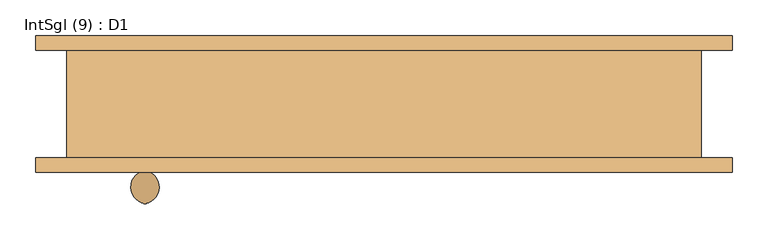
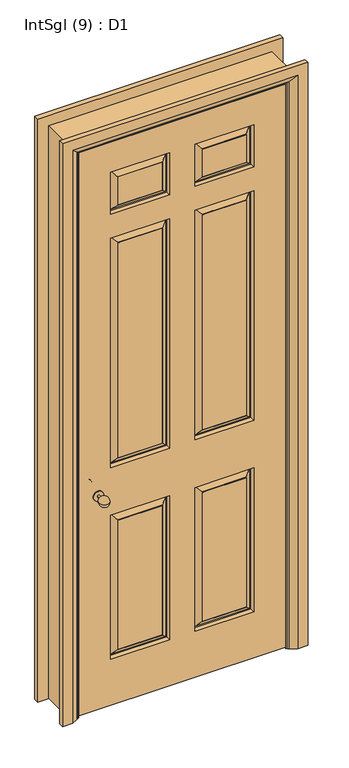
"""IFC4 building model written with IfcOpenShell, lengths in millimetres: door geometry, IntSgl (9) : D1."""

from ifc_helpers import new_model, si_unit, point, frame, origin, place, context, project, spatial, polyline, circle_curve, ellipse_curve, trimmed, outline, extrude, faceted_brep, source, transform, mapped, element, save
from ifc_brep_helpers import plane_surface, cylinder_surface, revolved_surface, advanced_brep


def intsgl_9_d1_ea64c5f3(model_context):
    return source(origin(), model_context, "Body", "SolidModel", [
        advanced_brep(
        [(-328.0, -18.0, 900.0), (-338.0, -18.0, 900.0), (-333.0, 26.437411, 900.0), (-328.0, -33.0, 900.0), (-338.0, -33.0, 900.0), (-353.0, -37.0, 900.0), (-313.0, -37.0, 900.0), (-353.0, -33.0, 900.0), (-313.0, -33.0, 900.0)],
        [
            (0, 1, circle_curve(frame((-333.0, -18.0, 900.0), z_axis=(0.0, 1.0, 0.0), x_axis=(-1.0, 0.0, 0.0)), 5.0)),
            (1, 2, circle_curve(frame((-329.8115138, 3.5786495, 900.0), z_axis=(0.0, 0.0, -1.0), x_axis=(0.0, -1.0, 0.0)), 23.0800654)),
            (2, 0, circle_curve(frame((-336.1884862, 3.5786495, 900.0), z_axis=(0.0, 0.0, -1.0), x_axis=(0.0, -1.0, 0.0)), 23.0800654)),
            (1, 0, circle_curve(frame((-333.0, -18.0, 900.0), z_axis=(0.0, 1.0, 0.0), x_axis=(-1.0, 0.0, 0.0)), 5.0)),
            (0, 3),
            (3, 4, circle_curve(frame((-333.0, -33.0, 900.0), z_axis=(0.0, 1.0, 0.0), x_axis=(-1.0, 0.0, 0.0)), 5.0)),
            (4, 1),
            (4, 3, circle_curve(frame((-333.0, -33.0, 900.0), z_axis=(0.0, 1.0, 0.0), x_axis=(-1.0, 0.0, 0.0)), 5.0)),
            (5, 6, circle_curve(frame((-333.0, -37.0, 900.0), z_axis=(0.0, -1.0, 0.0), x_axis=(1.0, 0.0, 0.0)), 20.0)),
            (6, 5, circle_curve(frame((-333.0, -37.0, 900.0), z_axis=(0.0, -1.0, 0.0), x_axis=(1.0, 0.0, 0.0)), 20.0)),
            (7, 8, circle_curve(frame((-333.0, -33.0, 900.0), z_axis=(0.0, 1.0, 0.0), x_axis=(1.0, 0.0, 0.0)), 20.0)),
            (8, 7, circle_curve(frame((-333.0, -33.0, 900.0), z_axis=(0.0, 1.0, 0.0), x_axis=(1.0, 0.0, 0.0)), 20.0)),
            (5, 7),
            (8, 6),
        ],
        [
            revolved_surface(trimmed(ellipse_curve(frame((-329.8115138, 3.5786495, 900.0), z_axis=(0.0, 0.0, 1.0), x_axis=(0.0, -1.0, 0.0)), 23.0800654, 23.0800654), [point((-333.0, 26.437411, 900.0))], [point((-338.0, -18.0, 900.0))], True, "CARTESIAN"), (-333.0, -33.0, 900.0), (0.0, -1.0, 0.0)),
            cylinder_surface(frame((-333.0, -33.0, 900.0), z_axis=(0.0, -1.0, 0.0), x_axis=(-1.0, 0.0, 0.0)), 5.0),
            plane_surface(frame((-313.0, -37.0, 900.0), z_axis=(0.0, -1.0, 0.0), x_axis=(0.0, 0.0, 1.0))),
            plane_surface(frame((-313.0, -33.0, 900.0), z_axis=(0.0, 1.0, 0.0), x_axis=(0.0, 0.0, -1.0))),
            cylinder_surface(frame((-333.0, -33.0, 900.0), z_axis=(0.0, -1.0, 0.0), x_axis=(1.0, 0.0, 0.0)), 20.0),
        ],
        [
            (0, [[1, 2, 3]]),
            (0, [[-2, 4, -3]]),
            (1, [[-1, 5, 6, 7]]),
            (1, [[-4, -7, 8, -5]]),
            (2, [[9, 10]]),
            (3, [[11, 12], [-6, -8]]),
            (4, [[-9, 13, -12, 14]]),
            (4, [[-10, -14, -11, -13]]),
        ],
    ),
        advanced_brep(
        [(-328.0, -94.0, 900.0), (-333.0, -138.437411, 900.0), (-338.0, -94.0, 900.0), (-338.0, -79.0, 900.0), (-328.0, -79.0, 900.0), (-353.0, -75.0, 900.0), (-313.0, -75.0, 900.0), (-353.0, -79.0, 900.0), (-313.0, -79.0, 900.0)],
        [
            (0, 1, circle_curve(frame((-336.1884862, -115.5786495, 900.0), z_axis=(0.0, 0.0, -1.0), x_axis=(0.0, 1.0, 0.0)), 23.0800654)),
            (1, 2, circle_curve(frame((-329.8115138, -115.5786495, 900.0), z_axis=(0.0, 0.0, -1.0), x_axis=(0.0, 1.0, 0.0)), 23.0800654)),
            (2, 0, circle_curve(frame((-333.0, -94.0, 900.0), z_axis=(0.0, -1.0, 0.0), x_axis=(-1.0, 0.0, 0.0)), 5.0)),
            (0, 2, circle_curve(frame((-333.0, -94.0, 900.0), z_axis=(0.0, -1.0, 0.0), x_axis=(-1.0, 0.0, 0.0)), 5.0)),
            (2, 3),
            (3, 4, circle_curve(frame((-333.0, -79.0, 900.0), z_axis=(0.0, -1.0, 0.0), x_axis=(-1.0, 0.0, 0.0)), 5.0)),
            (4, 0),
            (4, 3, circle_curve(frame((-333.0, -79.0, 900.0), z_axis=(0.0, -1.0, 0.0), x_axis=(-1.0, 0.0, 0.0)), 5.0)),
            (5, 6, circle_curve(frame((-333.0, -75.0, 900.0), z_axis=(0.0, 1.0, 0.0), x_axis=(1.0, 0.0, 0.0)), 20.0)),
            (6, 5, circle_curve(frame((-333.0, -75.0, 900.0), z_axis=(0.0, 1.0, 0.0), x_axis=(1.0, 0.0, 0.0)), 20.0)),
            (7, 8, circle_curve(frame((-333.0, -79.0, 900.0), z_axis=(0.0, -1.0, 0.0), x_axis=(1.0, 0.0, 0.0)), 20.0)),
            (8, 7, circle_curve(frame((-333.0, -79.0, 900.0), z_axis=(0.0, -1.0, 0.0), x_axis=(1.0, 0.0, 0.0)), 20.0)),
            (6, 8),
            (7, 5),
        ],
        [
            revolved_surface(trimmed(ellipse_curve(frame((-329.8115138, -115.5786495, 900.0), z_axis=(0.0, 0.0, -1.0), x_axis=(0.0, 1.0, 0.0)), 23.0800654, 23.0800654), [point((-333.0, -138.437411, 900.0))], [point((-338.0, -94.0, 900.0))], True, "CARTESIAN"), (-333.0, -79.0, 900.0), (0.0, 1.0, 0.0)),
            cylinder_surface(frame((-333.0, -79.0, 900.0), z_axis=(0.0, 1.0, 0.0), x_axis=(-1.0, 0.0, 0.0)), 5.0),
            plane_surface(frame((-313.0, -75.0, 900.0), z_axis=(0.0, 1.0, 0.0), x_axis=(0.0, 0.0, 1.0))),
            plane_surface(frame((-313.0, -79.0, 900.0), z_axis=(0.0, -1.0, 0.0), x_axis=(0.0, 0.0, -1.0))),
            cylinder_surface(frame((-333.0, -79.0, 900.0), z_axis=(0.0, 1.0, 0.0), x_axis=(1.0, 0.0, 0.0)), 20.0),
        ],
        [
            (0, [[1, 2, 3]]),
            (0, [[-1, 4, -2]]),
            (1, [[5, 6, 7, -3]]),
            (1, [[-7, 8, -5, -4]]),
            (2, [[9, 10]]),
            (3, [[11, 12], [-8, -6]]),
            (4, [[13, -11, 14, -10]]),
            (4, [[-14, -12, -13, -9]]),
        ],
    ),
        faceted_brep([(-408.0, -37.0, 2358.0), (408.0, -37.0, 2358.0), (408.0, -37.0, 8.0), (-408.0, -37.0, 8.0), (-50.0, -37.0, 800.0), (-283.0, -37.0, 800.0), (-283.0, -37.0, 200.0), (-50.0, -37.0, 200.0), (283.0, -37.0, 800.0), (50.0, -37.0, 800.0), (50.0, -37.0, 200.0), (283.0, -37.0, 200.0), (-50.0, -37.0, 1958.0), (-283.0, -37.0, 1958.0), (-283.0, -37.0, 1000.0), (-50.0, -37.0, 1000.0), (283.0, -37.0, 1958.0), (50.0, -37.0, 1958.0), (50.0, -37.0, 1000.0), (283.0, -37.0, 1000.0), (-50.0, -37.0, 2233.0), (-283.0, -37.0, 2233.0), (-283.0, -37.0, 2058.0), (-50.0, -37.0, 2058.0), (283.0, -37.0, 2233.0), (50.0, -37.0, 2233.0), (50.0, -37.0, 2058.0), (283.0, -37.0, 2058.0), (-80.0, -37.0, 230.0), (-253.0, -37.0, 230.0), (-253.0, -37.0, 770.0), (-80.0, -37.0, 770.0), (253.0, -37.0, 230.0), (80.0, -37.0, 230.0), (80.0, -37.0, 770.0), (253.0, -37.0, 770.0), (-80.0, -37.0, 1030.0), (-253.0, -37.0, 1030.0), (-253.0, -37.0, 1928.0), (-80.0, -37.0, 1928.0), (253.0, -37.0, 1030.0), (80.0, -37.0, 1030.0), (80.0, -37.0, 1928.0), (253.0, -37.0, 1928.0), (-80.0, -37.0, 2088.0), (-253.0, -37.0, 2088.0), (-253.0, -37.0, 2203.0), (-80.0, -37.0, 2203.0), (253.0, -37.0, 2088.0), (80.0, -37.0, 2088.0), (80.0, -37.0, 2203.0), (253.0, -37.0, 2203.0), (-408.0, -75.0, 2358.0), (-408.0, -75.0, 8.0), (408.0, -75.0, 8.0), (408.0, -75.0, 2358.0), (50.0, -75.0, 800.0), (283.0, -75.0, 800.0), (283.0, -75.0, 200.0), (50.0, -75.0, 200.0), (-283.0, -75.0, 800.0), (-50.0, -75.0, 800.0), (-50.0, -75.0, 200.0), (-283.0, -75.0, 200.0), (50.0, -75.0, 1958.0), (283.0, -75.0, 1958.0), (283.0, -75.0, 1000.0), (50.0, -75.0, 1000.0), (-283.0, -75.0, 1958.0), (-50.0, -75.0, 1958.0), (-50.0, -75.0, 1000.0), (-283.0, -75.0, 1000.0), (50.0, -75.0, 2233.0), (283.0, -75.0, 2233.0), (283.0, -75.0, 2058.0), (50.0, -75.0, 2058.0), (-283.0, -75.0, 2233.0), (-50.0, -75.0, 2233.0), (-50.0, -75.0, 2058.0), (-283.0, -75.0, 2058.0), (80.0, -75.0, 230.0), (253.0, -75.0, 230.0), (253.0, -75.0, 770.0), (80.0, -75.0, 770.0), (-253.0, -75.0, 230.0), (-80.0, -75.0, 230.0), (-80.0, -75.0, 770.0), (-253.0, -75.0, 770.0), (80.0, -75.0, 1030.0), (253.0, -75.0, 1030.0), (253.0, -75.0, 1928.0), (80.0, -75.0, 1928.0), (-253.0, -75.0, 1030.0), (-80.0, -75.0, 1030.0), (-80.0, -75.0, 1928.0), (-253.0, -75.0, 1928.0), (80.0, -75.0, 2088.0), (253.0, -75.0, 2088.0), (253.0, -75.0, 2203.0), (80.0, -75.0, 2203.0), (-253.0, -75.0, 2088.0), (-80.0, -75.0, 2088.0), (-80.0, -75.0, 2203.0), (-253.0, -75.0, 2203.0), (80.0, -74.0, 230.0), (80.0, -74.0, 770.0), (58.0, -60.0, 208.0), (78.0, -74.0, 228.0), (78.0, -74.0, 772.0), (58.0, -60.0, 792.0), (53.0, -60.0, 203.0), (53.0, -60.0, 797.0), (253.0, -74.0, 770.0), (255.0, -74.0, 772.0), (275.0, -60.0, 792.0), (280.0, -60.0, 797.0), (253.0, -74.0, 230.0), (255.0, -74.0, 228.0), (275.0, -60.0, 208.0), (280.0, -60.0, 203.0), (-253.0, -74.0, 230.0), (-253.0, -74.0, 770.0), (-275.0, -60.0, 208.0), (-255.0, -74.0, 228.0), (-255.0, -74.0, 772.0), (-275.0, -60.0, 792.0), (-280.0, -60.0, 203.0), (-280.0, -60.0, 797.0), (-80.0, -74.0, 770.0), (-78.0, -74.0, 772.0), (-58.0, -60.0, 792.0), (-53.0, -60.0, 797.0), (-80.0, -74.0, 230.0), (-78.0, -74.0, 228.0), (-58.0, -60.0, 208.0), (-53.0, -60.0, 203.0), (80.0, -74.0, 1030.0), (80.0, -74.0, 1928.0), (58.0, -60.0, 1008.0), (78.0, -74.0, 1028.0), (78.0, -74.0, 1930.0), (58.0, -60.0, 1950.0), (53.0, -60.0, 1003.0), (53.0, -60.0, 1955.0), (253.0, -74.0, 1928.0), (255.0, -74.0, 1930.0), (275.0, -60.0, 1950.0), (280.0, -60.0, 1955.0), (253.0, -74.0, 1030.0), (255.0, -74.0, 1028.0), (275.0, -60.0, 1008.0), (280.0, -60.0, 1003.0), (-253.0, -74.0, 1030.0), (-253.0, -74.0, 1928.0), (-275.0, -60.0, 1008.0), (-255.0, -74.0, 1028.0), (-255.0, -74.0, 1930.0), (-275.0, -60.0, 1950.0), (-280.0, -60.0, 1003.0), (-280.0, -60.0, 1955.0), (-80.0, -74.0, 1928.0), (-78.0, -74.0, 1930.0), (-58.0, -60.0, 1950.0), (-53.0, -60.0, 1955.0), (-80.0, -74.0, 1030.0), (-78.0, -74.0, 1028.0), (-58.0, -60.0, 1008.0), (-53.0, -60.0, 1003.0), (80.0, -74.0, 2088.0), (80.0, -74.0, 2203.0), (58.0, -60.0, 2066.0), (78.0, -74.0, 2086.0), (78.0, -74.0, 2205.0), (58.0, -60.0, 2225.0), (53.0, -60.0, 2061.0), (53.0, -60.0, 2230.0), (253.0, -74.0, 2203.0), (255.0, -74.0, 2205.0), (275.0, -60.0, 2225.0), (280.0, -60.0, 2230.0), (253.0, -74.0, 2088.0), (255.0, -74.0, 2086.0), (275.0, -60.0, 2066.0), (280.0, -60.0, 2061.0), (-253.0, -74.0, 2088.0), (-253.0, -74.0, 2203.0), (-275.0, -60.0, 2066.0), (-255.0, -74.0, 2086.0), (-255.0, -74.0, 2205.0), (-275.0, -60.0, 2225.0), (-280.0, -60.0, 2061.0), (-280.0, -60.0, 2230.0), (-80.0, -74.0, 2203.0), (-78.0, -74.0, 2205.0), (-58.0, -60.0, 2225.0), (-53.0, -60.0, 2230.0), (-80.0, -74.0, 2088.0), (-78.0, -74.0, 2086.0), (-58.0, -60.0, 2066.0), (-53.0, -60.0, 2061.0), (-80.0, -38.0, 230.0), (-80.0, -38.0, 770.0), (-58.0, -52.0, 208.0), (-78.0, -38.0, 228.0), (-78.0, -38.0, 772.0), (-58.0, -52.0, 792.0), (-53.0, -52.0, 203.0), (-53.0, -52.0, 797.0), (-253.0, -38.0, 770.0), (-255.0, -38.0, 772.0), (-275.0, -52.0, 792.0), (-280.0, -52.0, 797.0), (-253.0, -38.0, 230.0), (-255.0, -38.0, 228.0), (-275.0, -52.0, 208.0), (-280.0, -52.0, 203.0), (253.0, -38.0, 230.0), (253.0, -38.0, 770.0), (275.0, -52.0, 208.0), (255.0, -38.0, 228.0), (255.0, -38.0, 772.0), (275.0, -52.0, 792.0), (280.0, -52.0, 203.0), (280.0, -52.0, 797.0), (80.0, -38.0, 770.0), (78.0, -38.0, 772.0), (58.0, -52.0, 792.0), (53.0, -52.0, 797.0), (80.0, -38.0, 230.0), (78.0, -38.0, 228.0), (58.0, -52.0, 208.0), (53.0, -52.0, 203.0), (-80.0, -38.0, 1030.0), (-80.0, -38.0, 1928.0), (-58.0, -52.0, 1008.0), (-78.0, -38.0, 1028.0), (-78.0, -38.0, 1930.0), (-58.0, -52.0, 1950.0), (-53.0, -52.0, 1003.0), (-53.0, -52.0, 1955.0), (-253.0, -38.0, 1928.0), (-255.0, -38.0, 1930.0), (-275.0, -52.0, 1950.0), (-280.0, -52.0, 1955.0), (-253.0, -38.0, 1030.0), (-255.0, -38.0, 1028.0), (-275.0, -52.0, 1008.0), (-280.0, -52.0, 1003.0), (253.0, -38.0, 1030.0), (253.0, -38.0, 1928.0), (275.0, -52.0, 1008.0), (255.0, -38.0, 1028.0), (255.0, -38.0, 1930.0), (275.0, -52.0, 1950.0), (280.0, -52.0, 1003.0), (280.0, -52.0, 1955.0), (80.0, -38.0, 1928.0), (78.0, -38.0, 1930.0), (58.0, -52.0, 1950.0), (53.0, -52.0, 1955.0), (80.0, -38.0, 1030.0), (78.0, -38.0, 1028.0), (58.0, -52.0, 1008.0), (53.0, -52.0, 1003.0), (-80.0, -38.0, 2088.0), (-80.0, -38.0, 2203.0), (-58.0, -52.0, 2066.0), (-78.0, -38.0, 2086.0), (-78.0, -38.0, 2205.0), (-58.0, -52.0, 2225.0), (-53.0, -52.0, 2061.0), (-53.0, -52.0, 2230.0), (-253.0, -38.0, 2203.0), (-255.0, -38.0, 2205.0), (-275.0, -52.0, 2225.0), (-280.0, -52.0, 2230.0), (-253.0, -38.0, 2088.0), (-255.0, -38.0, 2086.0), (-275.0, -52.0, 2066.0), (-280.0, -52.0, 2061.0), (253.0, -38.0, 2088.0), (253.0, -38.0, 2203.0), (275.0, -52.0, 2066.0), (255.0, -38.0, 2086.0), (255.0, -38.0, 2205.0), (275.0, -52.0, 2225.0), (280.0, -52.0, 2061.0), (280.0, -52.0, 2230.0), (80.0, -38.0, 2203.0), (78.0, -38.0, 2205.0), (58.0, -52.0, 2225.0), (53.0, -52.0, 2230.0), (80.0, -38.0, 2088.0), (78.0, -38.0, 2086.0), (58.0, -52.0, 2066.0), (53.0, -52.0, 2061.0)], [[[0, 1, 2, 3], [4, 5, 6, 7], [8, 9, 10, 11], [12, 13, 14, 15], [16, 17, 18, 19], [20, 21, 22, 23], [24, 25, 26, 27]], [[28, 29, 30, 31]], [[32, 33, 34, 35]], [[36, 37, 38, 39]], [[40, 41, 42, 43]], [[44, 45, 46, 47]], [[48, 49, 50, 51]], [[52, 53, 54, 55], [56, 57, 58, 59], [60, 61, 62, 63], [64, 65, 66, 67], [68, 69, 70, 71], [72, 73, 74, 75], [76, 77, 78, 79]], [[80, 81, 82, 83]], [[84, 85, 86, 87]], [[88, 89, 90, 91]], [[92, 93, 94, 95]], [[96, 97, 98, 99]], [[100, 101, 102, 103]], [[3, 53, 52, 0]], [[2, 54, 53, 3]], [[1, 55, 54, 2]], [[0, 52, 55, 1]], [[104, 80, 83, 105]], [[106, 107, 108, 109]], [[56, 59, 110, 111]], [[83, 82, 112, 105]], [[108, 113, 114, 109]], [[111, 115, 57, 56]], [[82, 81, 116, 112]], [[113, 117, 118, 114]], [[115, 119, 58, 57]], [[104, 116, 81, 80]], [[107, 117, 113, 108], [105, 112, 116, 104]], [[106, 118, 117, 107]], [[110, 119, 115, 111], [109, 114, 118, 106]], [[59, 58, 119, 110]], [[120, 84, 87, 121]], [[122, 123, 124, 125]], [[60, 63, 126, 127]], [[87, 86, 128, 121]], [[124, 129, 130, 125]], [[127, 131, 61, 60]], [[86, 85, 132, 128]], [[129, 133, 134, 130]], [[131, 135, 62, 61]], [[120, 132, 85, 84]], [[123, 133, 129, 124], [121, 128, 132, 120]], [[122, 134, 133, 123]], [[126, 135, 131, 127], [125, 130, 134, 122]], [[63, 62, 135, 126]], [[136, 88, 91, 137]], [[138, 139, 140, 141]], [[64, 67, 142, 143]], [[91, 90, 144, 137]], [[140, 145, 146, 141]], [[143, 147, 65, 64]], [[90, 89, 148, 144]], [[145, 149, 150, 146]], [[147, 151, 66, 65]], [[136, 148, 89, 88]], [[139, 149, 145, 140], [137, 144, 148, 136]], [[138, 150, 149, 139]], [[142, 151, 147, 143], [141, 146, 150, 138]], [[67, 66, 151, 142]], [[152, 92, 95, 153]], [[154, 155, 156, 157]], [[68, 71, 158, 159]], [[95, 94, 160, 153]], [[156, 161, 162, 157]], [[159, 163, 69, 68]], [[94, 93, 164, 160]], [[161, 165, 166, 162]], [[163, 167, 70, 69]], [[152, 164, 93, 92]], [[155, 165, 161, 156], [153, 160, 164, 152]], [[154, 166, 165, 155]], [[158, 167, 163, 159], [157, 162, 166, 154]], [[71, 70, 167, 158]], [[168, 96, 99, 169]], [[170, 171, 172, 173]], [[72, 75, 174, 175]], [[99, 98, 176, 169]], [[172, 177, 178, 173]], [[175, 179, 73, 72]], [[98, 97, 180, 176]], [[177, 181, 182, 178]], [[179, 183, 74, 73]], [[168, 180, 97, 96]], [[171, 181, 177, 172], [169, 176, 180, 168]], [[170, 182, 181, 171]], [[174, 183, 179, 175], [173, 178, 182, 170]], [[75, 74, 183, 174]], [[184, 100, 103, 185]], [[186, 187, 188, 189]], [[76, 79, 190, 191]], [[103, 102, 192, 185]], [[188, 193, 194, 189]], [[191, 195, 77, 76]], [[102, 101, 196, 192]], [[193, 197, 198, 194]], [[195, 199, 78, 77]], [[184, 196, 101, 100]], [[187, 197, 193, 188], [185, 192, 196, 184]], [[186, 198, 197, 187]], [[190, 199, 195, 191], [189, 194, 198, 186]], [[79, 78, 199, 190]], [[200, 28, 31, 201]], [[202, 203, 204, 205]], [[4, 7, 206, 207]], [[31, 30, 208, 201]], [[204, 209, 210, 205]], [[207, 211, 5, 4]], [[30, 29, 212, 208]], [[209, 213, 214, 210]], [[211, 215, 6, 5]], [[200, 212, 29, 28]], [[203, 213, 209, 204], [201, 208, 212, 200]], [[202, 214, 213, 203]], [[206, 215, 211, 207], [205, 210, 214, 202]], [[7, 6, 215, 206]], [[216, 32, 35, 217]], [[218, 219, 220, 221]], [[8, 11, 222, 223]], [[35, 34, 224, 217]], [[220, 225, 226, 221]], [[223, 227, 9, 8]], [[34, 33, 228, 224]], [[225, 229, 230, 226]], [[227, 231, 10, 9]], [[216, 228, 33, 32]], [[219, 229, 225, 220], [217, 224, 228, 216]], [[218, 230, 229, 219]], [[222, 231, 227, 223], [221, 226, 230, 218]], [[11, 10, 231, 222]], [[232, 36, 39, 233]], [[234, 235, 236, 237]], [[12, 15, 238, 239]], [[39, 38, 240, 233]], [[236, 241, 242, 237]], [[239, 243, 13, 12]], [[38, 37, 244, 240]], [[241, 245, 246, 242]], [[243, 247, 14, 13]], [[232, 244, 37, 36]], [[235, 245, 241, 236], [233, 240, 244, 232]], [[234, 246, 245, 235]], [[238, 247, 243, 239], [237, 242, 246, 234]], [[15, 14, 247, 238]], [[248, 40, 43, 249]], [[250, 251, 252, 253]], [[16, 19, 254, 255]], [[43, 42, 256, 249]], [[252, 257, 258, 253]], [[255, 259, 17, 16]], [[42, 41, 260, 256]], [[257, 261, 262, 258]], [[259, 263, 18, 17]], [[248, 260, 41, 40]], [[251, 261, 257, 252], [249, 256, 260, 248]], [[250, 262, 261, 251]], [[254, 263, 259, 255], [253, 258, 262, 250]], [[19, 18, 263, 254]], [[264, 44, 47, 265]], [[266, 267, 268, 269]], [[20, 23, 270, 271]], [[47, 46, 272, 265]], [[268, 273, 274, 269]], [[271, 275, 21, 20]], [[46, 45, 276, 272]], [[273, 277, 278, 274]], [[275, 279, 22, 21]], [[264, 276, 45, 44]], [[267, 277, 273, 268], [265, 272, 276, 264]], [[266, 278, 277, 267]], [[270, 279, 275, 271], [269, 274, 278, 266]], [[23, 22, 279, 270]], [[280, 48, 51, 281]], [[282, 283, 284, 285]], [[24, 27, 286, 287]], [[51, 50, 288, 281]], [[284, 289, 290, 285]], [[287, 291, 25, 24]], [[50, 49, 292, 288]], [[289, 293, 294, 290]], [[291, 295, 26, 25]], [[280, 292, 49, 48]], [[283, 293, 289, 284], [281, 288, 292, 280]], [[282, 294, 293, 283]], [[286, 295, 291, 287], [285, 290, 294, 282]], [[27, 26, 295, 286]]]),
        faceted_brep([(-410.0, -75.0, 0.0), (-442.0, -75.0, 0.0), (-442.0, 75.0, 0.0), (-410.0, 75.0, 0.0), (-410.0, 75.0, 2360.0), (-410.0, -75.0, 2360.0), (-442.0, 75.0, 2392.0), (-442.0, -75.0, 2392.0), (410.0, -75.0, 0.0), (410.0, 75.0, 0.0), (442.0, 75.0, 0.0), (442.0, -75.0, 0.0), (410.0, -75.0, 2360.0), (442.0, -75.0, 2392.0), (442.0, 75.0, 2392.0), (410.0, 75.0, 2360.0)], [[[0, 1, 2, 3]], [[3, 4, 5, 0]], [[2, 6, 4, 3]], [[1, 7, 6, 2]], [[0, 5, 7, 1]], [[8, 9, 10, 11]], [[12, 8, 11, 13]], [[13, 11, 10, 14]], [[14, 10, 9, 15]], [[15, 9, 8, 12]], [[4, 15, 12, 5]], [[6, 14, 15, 4]], [[7, 13, 14, 6]], [[5, 12, 13, 7]]]),
        extrude(outline(polyline([(0.0, -391.0), (2341.0, -391.0), (2341.0, 391.0), (0.0, 391.0), (0.0, 410.0), (2360.0, 410.0), (2360.0, -410.0), (0.0, -410.0), (0.0, -391.0)])), frame((0.0, -35.0, 0.0), z_axis=(0.0, 1.0, 0.0), x_axis=(0.0, 0.0, 1.0)), (0.0, 0.0, 1.0), 32.0),
        advanced_brep(
        [(-485.0, 95.0, 0.0), (-445.0, 95.0, 0.0), (-419.0, 81.0, 0.0), (-415.0, 75.0, 0.0), (-485.0, 75.0, 0.0), (-485.0, 75.0, 2435.0), (-485.0, 95.0, 2435.0), (-415.0, 75.0, 2365.0), (415.0, 75.0, 2365.0), (415.0, 75.0, 0.0), (485.0, 75.0, 0.0), (485.0, 75.0, 2435.0), (-419.0, 81.0, 2369.0), (-445.0, 95.0, 2395.0), (485.0, 95.0, 2435.0), (485.0, 95.0, 0.0), (445.0, 95.0, 0.0), (445.0, 95.0, 2395.0), (419.0, 81.0, 0.0), (419.0, 81.0, 2369.0)],
        [
            (0, 1),
            (1, 2),
            (2, 3, circle_curve(frame((-423.0, 74.0, 0.0), z_axis=(0.0, 0.0, -1.0), x_axis=(-1.0, 0.0, 0.0)), 8.0622577)),
            (3, 4),
            (4, 0),
            (4, 5),
            (5, 6),
            (6, 0),
            (3, 7),
            (7, 8),
            (8, 9),
            (9, 10),
            (10, 11),
            (11, 5),
            (2, 12),
            (12, 7, ellipse_curve(frame((-423.0, 74.0, 2373.0), z_axis=(-0.7071067811865475, 0.0, -0.7071067811865475), x_axis=(0.7071067811865474, 0.0, -0.7071067811865476)), 11.4017543, 8.0622577)),
            (1, 13),
            (13, 12),
            (6, 14),
            (14, 15),
            (15, 16),
            (16, 17),
            (17, 13),
            (10, 15),
            (14, 11),
            (9, 18, circle_curve(frame((423.0, 74.0, 0.0), z_axis=(0.0, 0.0, -1.0), x_axis=(1.0, 0.0, 0.0)), 8.0622577)),
            (18, 16),
            (19, 18),
            (8, 19, ellipse_curve(frame((423.0, 74.0, 2373.0), z_axis=(0.7071067811865475, 0.0, -0.7071067811865475), x_axis=(0.7071067811865474, 0.0, 0.7071067811865476)), 11.4017543, 8.0622577)),
            (19, 17),
            (12, 19),
        ],
        [
            plane_surface(frame((-415.0, 75.0, 0.0), z_axis=(0.0, 0.0, -1.0), x_axis=(0.0, 1.0, 0.0))),
            plane_surface(frame((-485.0, 95.0, 0.0), z_axis=(-1.0, 0.0, 0.0), x_axis=(0.0, 0.0, 1.0))),
            plane_surface(frame((-485.0, 75.0, 0.0), z_axis=(0.0, -1.0, 0.0), x_axis=(0.0, 0.0, 1.0))),
            cylinder_surface(frame((-423.0, 74.0, 0.0), z_axis=(0.0, 0.0, -1.0), x_axis=(-1.0, 0.0, 0.0)), 8.0622577),
            plane_surface(frame((-419.0, 81.0, 0.0), z_axis=(0.4740998230350183, 0.8804710999221749, 0.0), x_axis=(0.0, 0.0, 1.0))),
            plane_surface(frame((-445.0, 95.0, 0.0), z_axis=(0.0, 1.0, 0.0), x_axis=(0.0, 0.0, 1.0))),
            plane_surface(frame((485.0, 95.0, 2435.0), z_axis=(1.0, 0.0, 0.0), x_axis=(0.0, 0.0, -1.0))),
            plane_surface(frame((415.0, 75.0, 0.0), z_axis=(0.0, 0.0, -1.0), x_axis=(0.0, 1.0, 0.0))),
            cylinder_surface(frame((423.0, 74.0, 2365.0), z_axis=(0.0, 0.0, 1.0), x_axis=(1.0, 0.0, 0.0)), 8.0622577),
            plane_surface(frame((419.0, 81.0, 2369.0), z_axis=(-0.4740998230350183, 0.8804710999221749, 0.0), x_axis=(0.0, 0.0, -1.0))),
            plane_surface(frame((-485.0, 95.0, 2435.0), z_axis=(0.0, 0.0, 1.0), x_axis=(1.0, 0.0, 0.0))),
            cylinder_surface(frame((-415.0, 74.0, 2373.0), z_axis=(-1.0, 0.0, 0.0), x_axis=(0.0, 0.0, 1.0)), 8.0622577),
            plane_surface(frame((-419.0, 81.0, 2369.0), z_axis=(0.0, 0.8804710999221749, -0.4740998230350183), x_axis=(1.0, 0.0, 0.0))),
        ],
        [
            (0, [[1, 2, 3, 4, 5]]),
            (1, [[6, 7, 8, -5]]),
            (2, [[9, 10, 11, 12, 13, 14, -6, -4]]),
            (3, [[15, 16, -9, -3]]),
            (4, [[17, 18, -15, -2]]),
            (5, [[-8, 19, 20, 21, 22, 23, -17, -1]]),
            (6, [[-13, 24, -20, 25]]),
            (7, [[-24, -12, 26, 27, -21]]),
            (8, [[28, -26, -11, 29]]),
            (9, [[-22, -27, -28, 30]]),
            (10, [[-14, -25, -19, -7]]),
            (11, [[31, -29, -10, -16]]),
            (12, [[-23, -30, -31, -18]]),
        ],
    ),
        advanced_brep(
        [(485.0, -95.0, 0.0), (445.0, -95.0, 0.0), (419.0, -81.0, 0.0), (415.0, -75.0, 0.0), (485.0, -75.0, 0.0), (485.0, -75.0, 2435.0), (485.0, -95.0, 2435.0), (415.0, -75.0, 2365.0), (-415.0, -75.0, 2365.0), (-415.0, -75.0, 0.0), (-485.0, -75.0, 0.0), (-485.0, -75.0, 2435.0), (419.0, -81.0, 2369.0), (445.0, -95.0, 2395.0), (-485.0, -95.0, 2435.0), (-485.0, -95.0, 0.0), (-445.0, -95.0, 0.0), (-445.0, -95.0, 2395.0), (-419.0, -81.0, 0.0), (-419.0, -81.0, 2369.0)],
        [
            (0, 1),
            (1, 2),
            (2, 3, circle_curve(frame((423.0, -74.0, 0.0), z_axis=(0.0, 0.0, -1.0), x_axis=(1.0, 0.0, 0.0)), 8.0622577)),
            (3, 4),
            (4, 0),
            (4, 5),
            (5, 6),
            (6, 0),
            (3, 7),
            (7, 8),
            (8, 9),
            (9, 10),
            (10, 11),
            (11, 5),
            (2, 12),
            (12, 7, ellipse_curve(frame((423.0, -74.0, 2373.0), z_axis=(0.7071067811865475, 0.0, -0.7071067811865475), x_axis=(-0.7071067811865474, 0.0, -0.7071067811865476)), 11.4017543, 8.0622577)),
            (1, 13),
            (13, 12),
            (6, 14),
            (14, 15),
            (15, 16),
            (16, 17),
            (17, 13),
            (10, 15),
            (14, 11),
            (9, 18, circle_curve(frame((-423.0, -74.0, 0.0), z_axis=(0.0, 0.0, -1.0), x_axis=(-1.0, 0.0, 0.0)), 8.0622577)),
            (18, 16),
            (19, 18),
            (8, 19, ellipse_curve(frame((-423.0, -74.0, 2373.0), z_axis=(-0.7071067811865475, 0.0, -0.7071067811865475), x_axis=(-0.7071067811865474, 0.0, 0.7071067811865476)), 11.4017543, 8.0622577)),
            (19, 17),
            (12, 19),
        ],
        [
            plane_surface(frame((415.0, -75.0, 0.0), z_axis=(0.0, 0.0, -1.0), x_axis=(0.0, -1.0, 0.0))),
            plane_surface(frame((485.0, -95.0, 0.0), z_axis=(1.0, 0.0, 0.0), x_axis=(0.0, 0.0, 1.0))),
            plane_surface(frame((485.0, -75.0, 0.0), z_axis=(0.0, 1.0, 0.0), x_axis=(0.0, 0.0, 1.0))),
            cylinder_surface(frame((423.0, -74.0, 0.0), z_axis=(0.0, 0.0, -1.0), x_axis=(1.0, 0.0, 0.0)), 8.0622577),
            plane_surface(frame((419.0, -81.0, 0.0), z_axis=(-0.4740998230350183, -0.8804710999221749, 0.0), x_axis=(0.0, 0.0, 1.0))),
            plane_surface(frame((445.0, -95.0, 0.0), z_axis=(0.0, -1.0, 0.0), x_axis=(0.0, 0.0, 1.0))),
            plane_surface(frame((-485.0, -95.0, 2435.0), z_axis=(-1.0, 0.0, 0.0), x_axis=(0.0, 0.0, -1.0))),
            plane_surface(frame((-415.0, -75.0, 0.0), z_axis=(0.0, 0.0, -1.0), x_axis=(0.0, -1.0, 0.0))),
            cylinder_surface(frame((-423.0, -74.0, 2365.0), z_axis=(0.0, 0.0, 1.0), x_axis=(-1.0, 0.0, 0.0)), 8.0622577),
            plane_surface(frame((-419.0, -81.0, 2369.0), z_axis=(0.4740998230350183, -0.8804710999221749, 0.0), x_axis=(0.0, 0.0, -1.0))),
            plane_surface(frame((485.0, -95.0, 2435.0), z_axis=(0.0, 0.0, 1.0), x_axis=(-1.0, 0.0, 0.0))),
            cylinder_surface(frame((415.0, -74.0, 2373.0), z_axis=(1.0, 0.0, 0.0), x_axis=(0.0, 0.0, 1.0)), 8.0622577),
            plane_surface(frame((419.0, -81.0, 2369.0), z_axis=(0.0, -0.8804710999221749, -0.4740998230350183), x_axis=(-1.0, 0.0, 0.0))),
        ],
        [
            (0, [[1, 2, 3, 4, 5]]),
            (1, [[6, 7, 8, -5]]),
            (2, [[9, 10, 11, 12, 13, 14, -6, -4]]),
            (3, [[15, 16, -9, -3]]),
            (4, [[17, 18, -15, -2]]),
            (5, [[-8, 19, 20, 21, 22, 23, -17, -1]]),
            (6, [[-13, 24, -20, 25]]),
            (7, [[-24, -12, 26, 27, -21]]),
            (8, [[28, -26, -11, 29]]),
            (9, [[-22, -27, -28, 30]]),
            (10, [[-14, -25, -19, -7]]),
            (11, [[31, -29, -10, -16]]),
            (12, [[-23, -30, -31, -18]]),
        ],
    ),
    ])


if __name__ == "__main__":
    model = new_model("IFC4")
    model_context = context("Model", 3, world=origin())
    ifc_project = project(units=[si_unit("LENGTHUNIT", "METRE", prefix="MILLI")], contexts=[model_context])
    site = spatial("IfcSite", under=ifc_project)
    building = spatial("IfcBuilding", under=site)
    placement = place(None, origin())
    intsgl_9_d1_shape = intsgl_9_d1_ea64c5f3(model_context)
    element("IfcDoor", 1, ObjectType="IntSgl (9) : D1", at=placement, inside=building, context=model_context, shape_type="MappedRepresentation", body=[
        mapped(intsgl_9_d1_shape, transform((0.0, 0.0, 0.0), x_axis=(1.0, 0.0, 0.0), y_axis=(0.0, 1.0, 0.0), z_axis=(0.0, 0.0, 1.0))),
    ])
    save(model, "model.ifc")

# Revit data of these elements
# Type "IntSgl (9) : D1"
#   Type Mark = "49"
#   Operation = "SingleSwingRight"
#   Manufacturer = "Revit"
#   Keynote = "L20"
#   UnderCut = 8 mm
#   Tolerance = 2 mm
#   Thickness = 38 mm
#   Structural Tolerance = 8 mm
#   StopDepth = 32 mm
#   Stop Thickness = 19 mm
#   Stile Top Rail = 125 mm
#   Stile Shutting = 125 mm
#   Stile Muntin Rail = 100 mm
#   Stile Lock Rail = 200 mm
#   Stile Intermediate/Frieze = 100 mm
#   Stile Hanging = 125 mm
#   Stile Bottom Rail = 200 mm
#   Rough Width = 900 mm
#   Rough Height = 2400 mm
#   Height to Top Lock Rail = 1000 mm
#   Handle Z Distance = 900 mm
#   Handle X Distance = 75 mm
#   Frame Thickness = 32 mm
#   Door Panel Width = 816 mm
#   Height = 2400 mm
#   Width = 900 mm
#   Door Panel Thickness = 38 mm
#   Door Panel Offset = 0 mm
#   Door Panel Height = 2350 mm
#   Architrave Setback = 5 mm
#   Vis - Ironmongery = yes
#   Material Ironmongery = Door - Handle
#   Material Frame = Door - Frame/Mullion
#   Material Door = Door - Panel
#   Material Architrave = Door - Architrave
#   Function = (empty or 0)
#   Wall Closure = (empty or 0)
# Element 1 (IfcDoor, "IntSgl (9) : D1")
#   Materials on its faces: "Door - Panel", "Door - Architrave", "Door - Frame/Mullion", "Door - Handle"
# Materials
#   "Door - Handle": colour RGB 0 0 0, transparency 0, Keynote = "P21", Cost = 0, Export to IFC = 0
#   "Door - Frame/Mullion": class "Wood", colour RGB 212 179 113, transparency 0, Keynote = "L20", Cost = 0, Export to IFC = 0
#   "Door - Panel": class "Wood", colour RGB 210 159 95, transparency 0, Keynote = "L20", Cost = 0, Export to IFC = 0
#   "Door - Architrave": class "Wood", colour RGB 154 90 5, transparency 0, Keynote = "P20", Cost = 0, Export to IFC = 0
